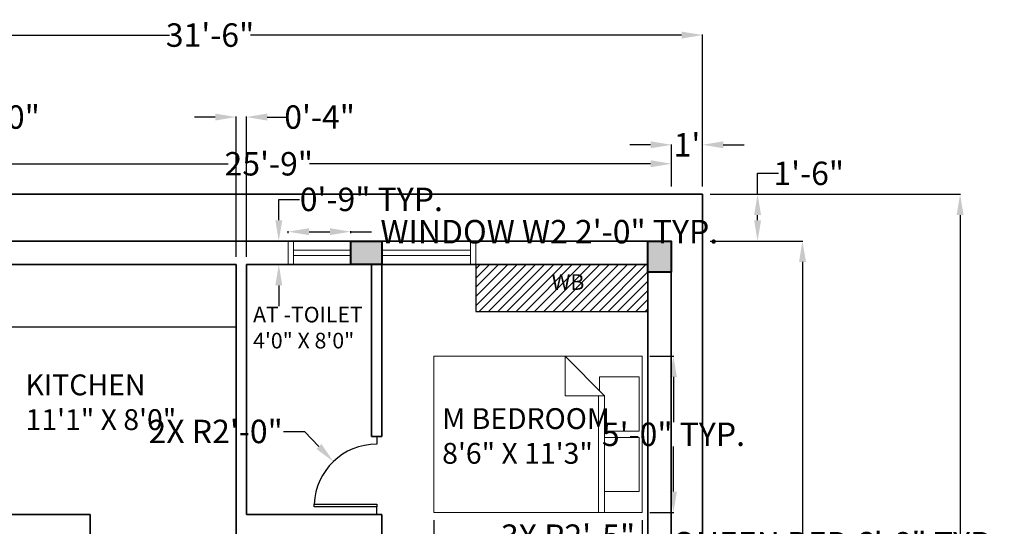
# Model space of a CAD drawing. Units: inches. Extents: x 411 to 983, y 289 to 833.
# Tile 3 of 3: x 605 to 983, y 639 to 833. Entities that reach past the tile are written whole.
import ezdxf

# ---------------------------------------------------------------- set-up
doc = ezdxf.new("R2010")
doc.units = ezdxf.units.IN
doc.header["$MEASUREMENT"] = 0
for name, color, linetype, lineweight in [('A-ANNO-DIMS', 2, 'Continuous', 18), ('A-ANNO-TEXT', 7, 'Continuous', 18), ('A-AREA-IDEN', 7, 'Continuous', 25), ('A-COLS', 18, 'Continuous', 40), ('A-DOOR', 4, 'Continuous', 25), ('A-FLOR-CASE', 2, 'Continuous', 25), ('A-FLOR-PATT', 3, 'Continuous', 13), ('A-FURN', 8, 'Continuous', 18), ('A-GLAZ', 4, 'Continuous', 18), ('A-WALL', 4, 'Continuous', 35), ('C-PROP', 4, 'Continuous', 35)]:
    doc.layers.add(name, color=color, linetype=linetype, lineweight=lineweight)
doc.layers.add('A-COLS-PATT', color=244, linetype='Continuous', lineweight=13, true_color=0x991b1e)
doc.styles.get("Standard").update_dxf_attribs({"font": 'arial.ttf'})
doc.dimstyles.get("Standard").update_dxf_attribs({"dimtxt": 9, "dimasz": 8, "dimexe": 0.18, "dimexo": 3, "dimgap": 0.09, "dimtad": 0, "dimtih": 1, "dimtoh": 1, "dimdec": 0, "dimzin": 0, "dimdsep": 46, "dimlunit": 3, "dimtxsty": 'Standard', "dimcen": 0.09, "dimadec": 0, "dimazin": 0, "dimtfac": 1, "dimtdec": 0, "dimtofl": 0, "dimtmove": 0, "dimatfit": 3, "dimfxl": 1, "dimtolj": 1, "dimtzin": 0, "dimarcsym": 0})

# ---------------------------------------------------------------- blocks, each defined once
blk = doc.blocks.new('*D9')
at = {"layer": 'A-ANNO-DIMS', "color": 0, "lineweight": -2, "transparency": 16777216}
for p, q in [((888.3, 766.4), (888.3, 774.4)), ((888.3, 774.4), (896.3, 774.4)), ((870.14, 766.4), (888.48, 766.4)), ((888.3, 756.4), (888.3, 758.4)), ((870.14, 748.4), (888.48, 748.4))]:
    blk.add_line(p, q, dxfattribs=at)
at = {"layer": 'A-ANNO-DIMS', "color": 0, "transparency": 16777216}
for points in [[(886.97, 758.4), (889.63, 758.4), (888.3, 766.4)], [(886.97, 756.4), (889.63, 756.4), (888.3, 748.4)]]:
    blk.add_solid(points, dxfattribs=at)
at = {"layer": 'Defpoints', "color": 0, "transparency": 16777216}
for p in [(867.14, 766.4), (888.3, 766.4), (867.14, 748.4)]:
    blk.add_point(p, dxfattribs=at)
at = {"layer": 'A-ANNO-DIMS', "color": 0, "transparency": 16777216, "insert": (907.93, 774.4), "char_height": 9, "attachment_point": 5}
blk.add_mtext('\\A1;1\'-6"', dxfattribs=at)
blk = doc.blocks.new('*D10')
at = {"layer": 'A-ANNO-DIMS', "color": 0, "lineweight": -2, "transparency": 16777216}
for p, q in [((870.14, 748.4), (905.71, 748.4)), ((905.53, 740.4), (905.53, 552.59)), ((905.53, 355.4), (905.53, 543.21)), ((870.14, 347.4), (905.71, 347.4))]:
    blk.add_line(p, q, dxfattribs=at)
at = {"layer": 'A-ANNO-DIMS', "color": 0, "transparency": 16777216}
for points in [[(904.2, 740.4), (906.87, 740.4), (905.53, 748.4)], [(904.2, 355.4), (906.87, 355.4), (905.53, 347.4)]]:
    blk.add_solid(points, dxfattribs=at)
at = {"layer": 'Defpoints', "color": 0, "transparency": 16777216}
for p in [(867.14, 748.4), (867.14, 347.4), (905.53, 347.4)]:
    blk.add_point(p, dxfattribs=at)
at = {"layer": 'A-ANNO-DIMS', "color": 0, "transparency": 16777216, "insert": (905.53, 547.9), "char_height": 9, "attachment_point": 5}
blk.add_mtext('\\A1;33\'-5"', dxfattribs=at)
blk = doc.blocks.new('*D11')
at = {"layer": 'A-ANNO-DIMS', "color": 0, "lineweight": -2, "transparency": 16777216}
for p, q in [((870.14, 766.4), (966.2, 766.4)), ((966.02, 758.4), (966.02, 552.59)), ((966.02, 337.4), (966.02, 543.21)), ((870.14, 329.4), (966.2, 329.4))]:
    blk.add_line(p, q, dxfattribs=at)
at = {"layer": 'A-ANNO-DIMS', "color": 0, "transparency": 16777216}
for points in [[(964.69, 758.4), (967.36, 758.4), (966.02, 766.4)], [(964.69, 337.4), (967.36, 337.4), (966.02, 329.4)]]:
    blk.add_solid(points, dxfattribs=at)
at = {"layer": 'Defpoints', "color": 0, "transparency": 16777216}
for p in [(867.14, 766.4), (966.02, 766.4), (867.14, 329.4)]:
    blk.add_point(p, dxfattribs=at)
at = {"layer": 'A-ANNO-DIMS', "color": 0, "transparency": 16777216, "insert": (966.02, 547.9), "char_height": 9, "attachment_point": 5}
blk.add_mtext('\\A1;36\'-5"', dxfattribs=at)
blk = doc.blocks.new('*D12')
at = {"layer": 'A-ANNO-DIMS', "color": 0, "lineweight": -2, "transparency": 16777216}
for p, q in [((847.25, 785.35), (839.25, 785.35)), ((855.25, 769.4), (855.25, 785.53)), ((867.14, 769.4), (867.14, 785.53)), ((875.14, 785.35), (883.14, 785.35))]:
    blk.add_line(p, q, dxfattribs=at)
at = {"layer": 'A-ANNO-DIMS', "color": 0, "transparency": 16777216}
for points in [[(847.25, 786.68), (847.25, 784.01), (855.25, 785.35)], [(875.14, 786.68), (875.14, 784.01), (867.14, 785.35)]]:
    blk.add_solid(points, dxfattribs=at)
at = {"layer": 'Defpoints', "color": 0, "transparency": 16777216}
for p in [(855.25, 785.35), (855.25, 766.4), (867.14, 766.4)]:
    blk.add_point(p, dxfattribs=at)
at = {"layer": 'A-ANNO-DIMS', "color": 0, "transparency": 16777216, "insert": (861.2, 785.35), "char_height": 9, "attachment_point": 5}
blk.add_mtext("\\A1;1'", dxfattribs=at)
blk = doc.blocks.new('*D13')
at = {"layer": 'A-ANNO-DIMS', "color": 0, "lineweight": -2, "transparency": 16777216}
for p, q in [((489.14, 769.4), (489.14, 827.65)), ((867.14, 769.4), (867.14, 827.65)), ((497.14, 827.47), (662.6, 827.47)), ((859.14, 827.47), (693.69, 827.47))]:
    blk.add_line(p, q, dxfattribs=at)
at = {"layer": 'A-ANNO-DIMS', "color": 0, "transparency": 16777216}
for points in [[(497.14, 828.81), (497.14, 826.14), (489.14, 827.47)], [(859.14, 828.81), (859.14, 826.14), (867.14, 827.47)]]:
    blk.add_solid(points, dxfattribs=at)
at = {"layer": 'Defpoints', "color": 0, "transparency": 16777216}
for p in [(489.14, 827.47), (489.14, 766.4), (867.14, 766.4)]:
    blk.add_point(p, dxfattribs=at)
at = {"layer": 'A-ANNO-DIMS', "color": 0, "transparency": 16777216, "insert": (678.14, 827.47), "char_height": 9, "attachment_point": 5}
blk.add_mtext('\\A1;31\'-6"', dxfattribs=at)
blk = doc.blocks.new('*D14')
at = {"layer": 'A-ANNO-DIMS', "color": 0, "lineweight": -2, "transparency": 16777216}
for p, q in [((546.14, 769.4), (546.14, 778.25)), ((554.14, 778.07), (685.07, 778.07)), ((847.25, 778.07), (716.32, 778.07)), ((855.25, 769.4), (855.25, 778.25))]:
    blk.add_line(p, q, dxfattribs=at)
at = {"layer": 'A-ANNO-DIMS', "color": 0, "transparency": 16777216}
for points in [[(554.14, 779.41), (554.14, 776.74), (546.14, 778.07)], [(847.25, 779.41), (847.25, 776.74), (855.25, 778.07)]]:
    blk.add_solid(points, dxfattribs=at)
at = {"layer": 'Defpoints', "color": 0, "transparency": 16777216}
for p in [(546.14, 778.07), (546.14, 766.4), (855.25, 766.4)]:
    blk.add_point(p, dxfattribs=at)
at = {"layer": 'A-ANNO-DIMS', "color": 0, "transparency": 16777216, "insert": (700.7, 778.07), "char_height": 9, "attachment_point": 5}
blk.add_mtext('\\A1;25\'-9"', dxfattribs=at)
blk = doc.blocks.new('*D16')
at = {"layer": 'A-ANNO-DIMS', "color": 0, "lineweight": -2, "transparency": 16777216}
for p, q in [((486.27, 765.55), (411.34, 743.26)), ((413.79, 735.64), (475.12, 529.5)), ((539.23, 313.98), (477.91, 520.12)), ((616.27, 328.55), (541.34, 306.26))]:
    blk.add_line(p, q, dxfattribs=at)
at = {"layer": 'A-ANNO-DIMS', "color": 0, "transparency": 16777216}
for points in [[(415.07, 736.02), (412.52, 735.26), (411.51, 743.31)], [(540.51, 314.36), (537.95, 313.6), (541.51, 306.31)]]:
    blk.add_solid(points, dxfattribs=at)
at = {"layer": 'Defpoints', "color": 0, "transparency": 16777216}
for p in [(489.14, 766.4), (411.51, 743.31), (619.14, 329.4)]:
    blk.add_point(p, dxfattribs=at)
at = {"layer": 'A-ANNO-DIMS', "color": 0, "transparency": 16777216, "insert": (476.51, 524.81), "char_height": 9, "attachment_point": 5}
blk.add_mtext("\\A1;38'", dxfattribs=at)
blk = doc.blocks.new('BED-QUEEN-60X80')
for p, q in [((0, 60), (0, 0)), ((80, 60), (0, 60)), ((50.4, 60), (65.6, 44.8)), ((50.4, 44.8), (50.4, 60)), ((80, 0), (80, 60)), ((63.6, 52), (63.6, 46.8)), ((78.8, 52), (63.6, 52)), ((78.8, 31.2), (78.8, 52)), ((65.6, 44.8), (50.4, 44.8)), ((63.2, 44.8), (63.2, 0)), ((65.6, 0), (65.6, 44.8)), ((65.6, 31.2), (78.8, 31.2)), ((78.8, 28.8), (65.6, 28.8)), ((78.8, 8), (78.8, 28.8)), ((65.6, 8), (78.8, 8)), ((0, 0), (80, 0))]:
    blk.add_line(p, q)
blk = doc.blocks.new('DOOR-SWING-30')
for p, q in [((3, 0), (3, 24)), ((3, 24), (4, 24)), ((4, 24), (4, 0)), ((0, 0), (3, 0)), ((4, 0), (3, 0)), ((30, 0), (27, 0))]:
    blk.add_line(p, q)
blk.add_arc((3.13, 0.15), 23.87, 359.6418, 87.9204)
blk = doc.blocks.new('WIN-36-POST')
for p, q in [((34, 0), (34, 9)), ((36, 0), (36, 9)), ((34, 5.5), (0, 5.5)), ((34, 3.5), (0, 3.5))]:
    blk.add_line(p, q)
blk = doc.blocks.new('WIN-24-POST')
for p, q in [((0, 9), (0, 0)), ((2, 9), (2, 0)), ((24, 5.5), (2, 5.5)), ((24, 3.5), (2, 3.5))]:
    blk.add_line(p, q)
blk = doc.blocks.new('*D36')
at = {"layer": 'A-ANNO-DIMS', "color": 0, "lineweight": -2, "transparency": 16777216}
for p, q in [((708.14, 751.4), (708.14, 752.18)), ((732.14, 751.4), (732.14, 752.18)), ((716.14, 752), (724.14, 752)), ((732.14, 752), (740.14, 752))]:
    blk.add_line(p, q, dxfattribs=at)
at = {"layer": 'A-ANNO-DIMS', "color": 0, "transparency": 16777216}
for points in [[(716.14, 753.34), (716.14, 750.67), (708.14, 752)], [(724.14, 753.34), (724.14, 750.67), (732.14, 752)]]:
    blk.add_solid(points, dxfattribs=at)
at = {"layer": 'Defpoints', "color": 0, "transparency": 16777216}
for p in [(708.14, 748.4), (732.14, 752), (732.14, 748.4)]:
    blk.add_point(p, dxfattribs=at)
at = {"layer": 'A-ANNO-DIMS', "color": 0, "transparency": 16777216, "insert": (808.35, 752), "char_height": 9, "attachment_point": 5}
blk.add_mtext('\\A1;WINDOW W2 2\'-0" TYP.', dxfattribs=at)
blk = doc.blocks.new('*D37')
at = {"layer": 'A-ANNO-DIMS', "color": 0, "lineweight": -2, "transparency": 16777216}
for p, q in [((704.54, 756.4), (704.54, 764.4)), ((704.54, 764.4), (712.54, 764.4)), ((705.14, 748.4), (704.36, 748.4)), ((705.14, 739.4), (704.36, 739.4)), ((704.54, 731.4), (704.54, 723.4))]:
    blk.add_line(p, q, dxfattribs=at)
at = {"layer": 'A-ANNO-DIMS', "color": 0, "transparency": 16777216}
for points in [[(703.21, 756.4), (705.88, 756.4), (704.54, 748.4)], [(703.21, 731.4), (705.88, 731.4), (704.54, 739.4)]]:
    blk.add_solid(points, dxfattribs=at)
at = {"layer": 'Defpoints', "color": 0, "transparency": 16777216}
for p in [(704.54, 748.4), (708.14, 748.4), (708.14, 739.4)]:
    blk.add_point(p, dxfattribs=at)
at = {"layer": 'A-ANNO-DIMS', "color": 0, "transparency": 16777216, "insert": (740.06, 764.4), "char_height": 9, "attachment_point": 5}
blk.add_mtext('\\A1;0\'-9" TYP.', dxfattribs=at)
blk = doc.blocks.new('*D40')
at = {"layer": 'A-ANNO-DIMS', "color": 0, "lineweight": -2, "transparency": 16777216}
for p, q in [((764, 641.23), (764, 632.05)), ((844, 641.23), (844, 632.05)), ((772, 632.23), (836, 632.23)), ((844, 632.23), (852, 632.23))]:
    blk.add_line(p, q, dxfattribs=at)
at = {"layer": 'A-ANNO-DIMS', "color": 0, "transparency": 16777216}
for points in [[(772, 633.56), (772, 630.89), (764, 632.23)], [(836, 633.56), (836, 630.89), (844, 632.23)]]:
    blk.add_solid(points, dxfattribs=at)
at = {"layer": 'Defpoints', "color": 0, "transparency": 16777216}
for p in [(764, 644.23), (844, 644.23), (844, 632.23)]:
    blk.add_point(p, dxfattribs=at)
at = {"layer": 'A-ANNO-DIMS', "color": 0, "transparency": 16777216, "insert": (918.29, 632.23), "char_height": 9, "attachment_point": 5}
blk.add_mtext('\\A1;QUEEN BED 6\'-8" TYP.', dxfattribs=at)
blk = doc.blocks.new('*D41')
at = {"layer": 'A-ANNO-DIMS', "color": 0, "lineweight": -2, "transparency": 16777216}
for p, q in [((847, 704.23), (856.18, 704.23)), ((856, 696.23), (856, 678.91)), ((856, 652.23), (856, 669.54)), ((847, 644.23), (856.18, 644.23))]:
    blk.add_line(p, q, dxfattribs=at)
at = {"layer": 'A-ANNO-DIMS', "color": 0, "transparency": 16777216}
for points in [[(854.67, 696.23), (857.34, 696.23), (856, 704.23)], [(854.67, 652.23), (857.34, 652.23), (856, 644.23)]]:
    blk.add_solid(points, dxfattribs=at)
at = {"layer": 'Defpoints', "color": 0, "transparency": 16777216}
for p in [(844, 704.23), (856, 704.23), (844, 644.23)]:
    blk.add_point(p, dxfattribs=at)
at = {"layer": 'A-ANNO-DIMS', "color": 0, "transparency": 16777216, "insert": (856, 674.23), "char_height": 9, "attachment_point": 5}
blk.add_mtext('\\A1;5\'-0" TYP.', dxfattribs=at)
blk = doc.blocks.new('*D44')
at = {"layer": 'A-ANNO-DIMS', "color": 0, "lineweight": -2, "transparency": 16777216}
for p, q in [((555.14, 742.4), (555.14, 796.18)), ((563.14, 796), (571.14, 796)), ((579.14, 718.4), (579.14, 796.18)), ((579.14, 796), (587.14, 796))]:
    blk.add_line(p, q, dxfattribs=at)
at = {"layer": 'A-ANNO-DIMS', "color": 0, "transparency": 16777216}
for points in [[(563.14, 797.34), (563.14, 794.67), (555.14, 796)], [(571.14, 797.34), (571.14, 794.67), (579.14, 796)]]:
    blk.add_solid(points, dxfattribs=at)
at = {"layer": 'Defpoints', "color": 0, "transparency": 16777216}
for p in [(579.14, 796), (555.14, 739.4), (579.14, 715.4)]:
    blk.add_point(p, dxfattribs=at)
at = {"layer": 'A-ANNO-DIMS', "color": 0, "transparency": 16777216, "insert": (599.27, 796), "char_height": 9, "attachment_point": 5}
blk.add_mtext('\\A1;2\'-0"', dxfattribs=at)
blk = doc.blocks.new('*D45')
at = {"layer": 'A-ANNO-DIMS', "color": 0, "lineweight": -2, "transparency": 16777216}
for p, q in [((680.14, 796), (672.14, 796)), ((688.14, 742.4), (688.14, 796.18)), ((692.14, 742.4), (692.14, 796.18)), ((700.14, 796), (708.14, 796))]:
    blk.add_line(p, q, dxfattribs=at)
at = {"layer": 'A-ANNO-DIMS', "color": 0, "transparency": 16777216}
for points in [[(680.14, 797.34), (680.14, 794.67), (688.14, 796)], [(700.14, 797.34), (700.14, 794.67), (692.14, 796)]]:
    blk.add_solid(points, dxfattribs=at)
at = {"layer": 'Defpoints', "color": 0, "transparency": 16777216}
for p in [(692.14, 796), (688.14, 739.4), (692.14, 739.4)]:
    blk.add_point(p, dxfattribs=at)
at = {"layer": 'A-ANNO-DIMS', "color": 0, "transparency": 16777216, "insert": (720.2, 796), "char_height": 9, "attachment_point": 5}
blk.add_mtext('\\A1;0\'-4"', dxfattribs=at)
blk = doc.blocks.new('*D47')
at = {"layer": 'A-ANNO-DIMS', "color": 0, "lineweight": -2, "transparency": 16777216}
for p, q in [((781.52, 635.12), (774.76, 628.58)), ((789.52, 635.12), (781.52, 635.12)), ((748.05, 602.85), (748.23, 602.85)), ((748.14, 602.76), (748.14, 602.94))]:
    blk.add_line(p, q, dxfattribs=at)
at = {"layer": 'A-ANNO-DIMS', "color": 0, "transparency": 16777216}
blk.add_solid([(773.83, 629.54), (775.68, 627.62), (769.01, 623.02)], dxfattribs=at)
at = {"layer": 'Defpoints', "color": 0, "transparency": 16777216}
for p in [(769.01, 623.02), (748.14, 602.85)]:
    blk.add_point(p, dxfattribs=at)
at = {"layer": 'A-ANNO-DIMS', "color": 0, "transparency": 16777216, "insert": (815.55, 635.12), "char_height": 9, "attachment_point": 5}
blk.add_mtext('\\A1;3X R2\'-5"', dxfattribs=at)
blk = doc.blocks.new('*D48')
at = {"layer": 'A-ANNO-DIMS', "color": 0, "lineweight": -2, "transparency": 16777216}
for p, q in [((706.41, 675.32), (714.41, 675.32)), ((714.41, 675.32), (719.95, 669.54)), ((741.9, 646.54), (742.08, 646.54)), ((741.99, 646.45), (741.99, 646.63))]:
    blk.add_line(p, q, dxfattribs=at)
at = {"layer": 'A-ANNO-DIMS', "color": 0, "transparency": 16777216}
blk.add_solid([(720.91, 670.47), (718.98, 668.62), (725.48, 663.77)], dxfattribs=at)
at = {"layer": 'Defpoints', "color": 0, "transparency": 16777216}
for p in [(725.48, 663.77), (741.99, 646.54)]:
    blk.add_point(p, dxfattribs=at)
at = {"layer": 'A-ANNO-DIMS', "color": 0, "transparency": 16777216, "insert": (680.31, 675.32), "char_height": 9, "attachment_point": 5}
blk.add_mtext('\\A1;2X R2\'-0"', dxfattribs=at)

msp = doc.modelspace()

# ---------------------------------------------------------------- hatches: boundary and pattern name
at = {"layer": 'A-COLS-PATT'}
h = msp.add_hatch(color=256, dxfattribs=at)
h.dxf.hatch_style = 1
h.paths.add_polyline_path([(625.14, 347.4), (625.14, 356.4), (615.14, 356.4), (615.14, 347.4)])
h.paths.add_polyline_path([(740.14, 347.4), (740.14, 356.4), (730.14, 356.4), (730.14, 347.4)])
h.paths.add_polyline_path([(740.14, 419.4), (749.14, 419.4), (749.14, 431.4), (740.14, 431.4)])
h.paths.add_polyline_path([(611.14, 419.4), (620.14, 419.4), (620.14, 431.4), (611.14, 431.4)])
h.paths.add_polyline_path([(846.14, 419.4), (855.14, 419.4), (855.14, 431.4), (846.14, 431.4)])
h.paths.add_polyline_path([(855.14, 612.4), (846.14, 612.4), (846.14, 600.4), (855.14, 600.4)])
h.paths.add_polyline_path([(744.14, 612.4), (735.14, 612.4), (735.14, 600.4), (744.14, 600.4)])
h.paths.add_polyline_path([(546.14, 634.4), (555.14, 634.4), (555.14, 646.4), (546.14, 646.4)])
h.paths.add_polyline_path([(555.14, 748.4), (546.14, 748.4), (546.14, 736.4), (555.14, 736.4)])
h.paths.add_polyline_path([(744.14, 748.4), (732.14, 748.4), (732.14, 739.4), (744.14, 739.4)])
h.paths.add_polyline_path([(855.14, 748.4), (846.14, 748.4), (846.14, 736.4), (855.14, 736.4)])
at = {"layer": 'A-FLOR-PATT'}
h = msp.add_hatch(dxfattribs=at)
h.set_pattern_fill('ANSI31', color=256, scale=20)
h.paths.add_polyline_path([(846.14, 739.4), (780.14, 739.4), (780.14, 721.4), (846.14, 721.4)])
h.paths.add_polyline_path([(846.14, 548.4), (814.14, 548.4), (814.14, 530.4), (846.14, 530.4)])
h.paths.add_polyline_path([(807.66, 726.4), (824.16, 726.4), (824.16, 738.76), (807.66, 738.76)], flags=24)
h.paths.add_polyline_path([(820.06, 534.9), (836.57, 534.9), (836.57, 547.26), (820.06, 547.26)], flags=24)

# ---------------------------------------------------------------- linework, layer by layer
at = {"layer": 'A-COLS'}
for points in [[(744.14, 739.4), (732.14, 739.4), (732.14, 748.4), (744.14, 748.4)], [(846.14, 748.4), (855.14, 748.4), (855.14, 736.4), (846.14, 736.4)]]:
    msp.add_lwpolyline(points, close=True, dxfattribs=at)
at = {"layer": 'A-FLOR-CASE'}
for p, q in [((780.14, 739.4), (780.14, 721.4)), ((780.14, 721.4), (846.14, 721.4)), ((688.14, 715.4), (579.14, 715.4))]:
    msp.add_line(p, q, dxfattribs=at)
at = {"layer": 'A-WALL'}
for p, q in [((855.14, 748.4), (546.14, 748.4)), ((855.14, 347.4), (855.14, 748.4)), ((688.14, 739.4), (555.14, 739.4)), ((688.14, 634.4), (688.14, 739.4)), ((692.14, 643.4), (692.14, 739.4)), ((740.14, 739.4), (692.14, 739.4)), ((740.14, 673.4), (740.14, 739.4)), ((846.14, 739.4), (744.14, 739.4)), ((744.14, 673.4), (744.14, 739.4)), ((846.14, 604.4), (846.14, 739.4)), ((744.14, 673.4), (740.14, 673.4)), ((632.14, 643.4), (555.14, 643.4)), ((632.14, 634.4), (632.14, 643.4)), ((744.14, 643.4), (692.14, 643.4)), ((744.14, 600.4), (744.14, 643.4))]:
    msp.add_line(p, q, dxfattribs=at)
at = {"layer": 'C-PROP'}
for p, q in [((867.14, 766.4), (489.14, 766.4)), ((867.14, 329.4), (867.14, 766.4))]:
    msp.add_line(p, q, dxfattribs=at)

# ---------------------------------------------------------------- block references
at = {"layer": 'A-DOOR', "rotation": 90.0000000000003}
msp.add_blockref('DOOR-SWING-30', (742.14, 643.4), dxfattribs=at)
at = {"layer": 'A-FURN'}
msp.add_blockref('BED-QUEEN-60X80', (764, 644.23), dxfattribs=at)
at = {"layer": 'A-GLAZ'}
for name, p in [('WIN-24-POST', (708.14, 739.4)), ('WIN-36-POST', (744.14, 739.4))]:
    msp.add_blockref(name, p, dxfattribs=at)

# ---------------------------------------------------------------- texts
at = {"layer": 'A-ANNO-TEXT', "insert": (809.26, 735.67), "char_height": 6, "attachment_point": 1}
msp.add_mtext_dynamic_manual_height_columns('WB', width=69.531, gutter_width=1, heights=[0], dxfattribs=at)
at = {"layer": 'A-AREA-IDEN', "attachment_point": 1}
for s, insert, char_height in [('AT -TOILET\\P4\'0" X 8\'0"', (694.67, 723.18), 6), ('KITCHEN\\P11\'1" X 8\'0"', (607.35, 697.19), 8), ('M BEDROOM\\P8\'6" X 11\'3"', (767.24, 684.25), 8)]:
    msp.add_mtext_dynamic_manual_height_columns(s, width=69.531, gutter_width=1, heights=[0], dxfattribs=dict(at, insert=insert, char_height=char_height))

# ---------------------------------------------------------------- dimensions: what is measured, and where the dimension line sits
at = {"layer": 'A-ANNO-DIMS'}
for base, p1, p2, override, picture, middle in [((489.14, 827.47), (867.14, 766.4), (489.14, 766.4), {"dimclrd": 0, "dimclre": 0, "dimclrt": 0}, '*D13', (678.14, 827.47)), ((579.14, 796), (555.14, 739.4), (579.14, 715.4), {"dimdec": 1, "dimlfac": 1, "dimrnd": 0, "dimzin": 1, "dimdsep": 46, "dimlunit": 4, "dimfrac": 2}, '*D44', (599.27, 796)), ((692.14, 796), (688.14, 739.4), (692.14, 739.4), {"dimdec": 1, "dimlfac": 1, "dimrnd": 0, "dimzin": 1, "dimdsep": 46, "dimlunit": 4, "dimfrac": 2}, '*D45', (720.2, 796)), ((855.25, 785.35), (867.14, 766.4), (855.25, 766.4), {"dimclrd": 0, "dimclre": 0, "dimclrt": 0}, '*D12', (861.2, 785.35)), ((546.14, 778.07), (855.25, 766.4), (546.14, 766.4), {"dimclrd": 0, "dimclre": 0, "dimclrt": 0}, '*D14', (700.7, 778.07))]:
    dim = msp.add_linear_dim(base=base, p1=p1, p2=p2, dimstyle='Standard', override=override, dxfattribs=at)
    dim.commit()
    dim.dimension.update_dxf_attribs({"geometry": picture, "text_midpoint": middle})
for base, p1, p2, text, picture, middle in [((732.14, 752), (708.14, 748.4), (732.14, 748.4), 'WINDOW W2 <> TYP.', '*D36', (808.35, 752)), ((844, 632.23), (764, 644.23), (844, 644.23), 'QUEEN BED <> TYP.', '*D40', (918.29, 632.23))]:
    dim = msp.add_linear_dim(base=base, p1=p1, p2=p2, text=text, dimstyle='Standard', override={"dimdec": 1, "dimlfac": 1, "dimrnd": 0, "dimzin": 1, "dimdsep": 46, "dimlunit": 4, "dimfrac": 2}, dxfattribs=at)
    dim.commit()
    dim.dimension.update_dxf_attribs({"geometry": picture, "text_midpoint": middle})
for base, p1, p2, picture, middle in [((888.3, 766.4), (867.14, 748.4), (867.14, 766.4), '*D9', (907.93, 774.4)), ((966.02, 766.4), (867.14, 329.4), (867.14, 766.4), '*D11', (966.02, 547.9)), ((905.53, 347.4), (867.14, 748.4), (867.14, 347.4), '*D10', (905.53, 547.9))]:
    dim = msp.add_linear_dim(base=base, p1=p1, p2=p2, angle=90, dimstyle='Standard', override={"dimclrd": 0, "dimclre": 0, "dimclrt": 0}, dxfattribs=at)
    dim.commit()
    dim.dimension.update_dxf_attribs({"geometry": picture, "text_midpoint": middle})
for base, p1, p2, picture, middle in [((704.54, 748.4), (708.14, 739.4), (708.14, 748.4), '*D37', (740.06, 764.4)), ((856, 704.23), (844, 644.23), (844, 704.23), '*D41', (856, 674.23))]:
    dim = msp.add_linear_dim(base=base, p1=p1, p2=p2, angle=90, text='<> TYP.', dimstyle='Standard', override={"dimdec": 1, "dimlfac": 1, "dimrnd": 0, "dimzin": 1, "dimdsep": 46, "dimlunit": 4, "dimfrac": 2}, dxfattribs=at)
    dim.commit()
    dim.dimension.update_dxf_attribs({"geometry": picture, "text_midpoint": middle})
dim = msp.add_aligned_dim(p1=(619.14, 329.4), p2=(489.14, 766.4), distance=80.99, dimstyle='Standard', override={"dimclrd": 0, "dimclre": 0, "dimclrt": 0}, dxfattribs=at)
dim.commit()
dim.dimension.update_dxf_attribs({"geometry": '*D16', "text_midpoint": (476.51, 524.81)})
dim = msp.add_radius_dim(center=(741.99, 646.54), mpoint=(725.48, 663.77), text='2X <>', dimstyle='Standard', override={"dimdec": 1, "dimlfac": 1, "dimrnd": 0, "dimzin": 1, "dimdsep": 46, "dimlunit": 4, "dimfrac": 2}, dxfattribs=at)
dim.commit()
dim.dimension.update_dxf_attribs({"geometry": '*D48', "text_midpoint": (680.31, 675.32)})
dim = msp.add_radius_dim(center=(748.14, 602.85), mpoint=(769.01, 623.02), text='3X <>', dimstyle='Standard', override={"dimdec": 1, "dimlfac": 1, "dimrnd": 0, "dimzin": 1, "dimdsep": 46, "dimlunit": 4, "dimfrac": 2}, dxfattribs=at)
dim.commit()
dim.dimension.update_dxf_attribs({"geometry": '*D47', "text_midpoint": (815.55, 635.12), "dimtype": 164})

doc.saveas('drawing.dxf')
